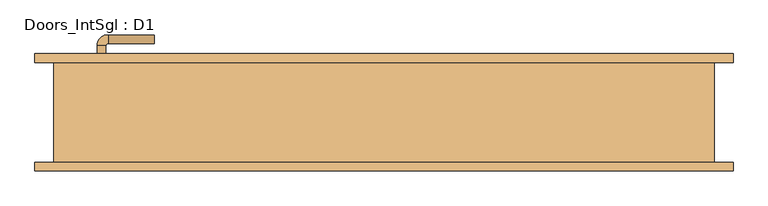
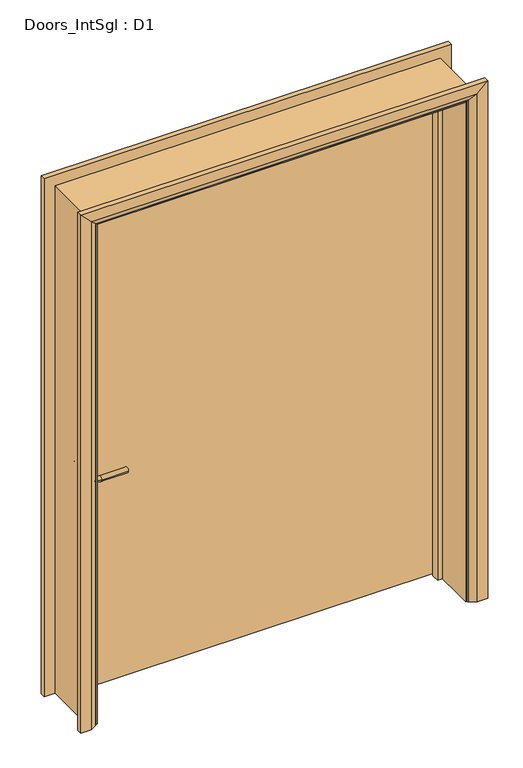
"""IFC4 building model written with IfcOpenShell, lengths in millimetres: door geometry, Doors_IntSgl : D1."""

from ifc_helpers import new_model, si_unit, point, frame, frame_2d, origin, place, context, project, spatial, polyline, circle_curve, ellipse_curve, trimmed, segment, composite_curve, outline, extrude, faceted_brep, source, transform, mapped, element, save
from ifc_brep_helpers import plane_surface, cylinder_surface, revolved_surface, advanced_brep


def doors_intsgl_d1_5c0f405e(model_context):
    return source(origin(), model_context, "Body", "SolidModel", [
        advanced_brep(
        [(-655.0, 68.3, 900.0), (-635.0, 68.3, 900.0), (-635.0, 38.3, 900.0), (-655.0, 38.3, 900.0), (-630.0, 33.3, 900.0), (-630.0, 13.3, 900.0), (-525.0, 13.3, 900.0), (-525.0, 33.3, 900.0)],
        [
            (0, 1, circle_curve(frame((-645.0, 68.3, 900.0), z_axis=(0.0, 1.0, 0.0), x_axis=(1.0, 0.0, 0.0)), 10.0)),
            (1, 0, circle_curve(frame((-645.0, 68.3, 900.0), z_axis=(0.0, 1.0, 0.0), x_axis=(1.0, 0.0, 0.0)), 10.0)),
            (1, 2),
            (2, 3, circle_curve(frame((-645.0, 38.3, 900.0), z_axis=(0.0, 1.0, 0.0), x_axis=(1.0, 0.0, 0.0)), 10.0)),
            (3, 0),
            (3, 2, circle_curve(frame((-645.0, 38.3, 900.0), z_axis=(0.0, 1.0, 0.0), x_axis=(1.0, 0.0, 0.0)), 10.0)),
            (4, 5, circle_curve(frame((-630.0, 23.3, 900.0), z_axis=(-1.0, 0.0, 0.0), x_axis=(0.0, 1.0, 0.0)), 10.0)),
            (5, 3, circle_curve(frame((-630.0, 38.3, 900.0), z_axis=(0.0, 0.0, -1.0), x_axis=(-1.0, 0.0, 0.0)), 25.0)),
            (2, 4, circle_curve(frame((-630.0, 38.3, 900.0), z_axis=(0.0, 0.0, 1.0), x_axis=(-1.0, 0.0, 0.0)), 5.0)),
            (5, 4, circle_curve(frame((-630.0, 23.3, 900.0), z_axis=(-1.0, 0.0, 0.0), x_axis=(0.0, 1.0, 0.0)), 10.0)),
            (6, 7, circle_curve(frame((-525.0, 23.3, 900.0), z_axis=(1.0, 0.0, 0.0), x_axis=(0.0, 1.0, 0.0)), 10.0)),
            (7, 6, circle_curve(frame((-525.0, 23.3, 900.0), z_axis=(1.0, 0.0, 0.0), x_axis=(0.0, 1.0, 0.0)), 10.0)),
            (4, 7),
            (6, 5),
        ],
        [
            plane_surface(frame((-645.0, 68.3, 900.0), z_axis=(0.0, 1.0, 0.0), x_axis=(0.0, 0.0, 1.0))),
            cylinder_surface(frame((-645.0, 68.3, 900.0), z_axis=(0.0, 1.0, 0.0), x_axis=(1.0, 0.0, 0.0)), 10.0),
            revolved_surface(trimmed(ellipse_curve(frame((-645.0, 38.3, 900.0), z_axis=(0.0, -1.0, 0.0), x_axis=(1.0, 0.0, 0.0)), 10.0, 10.0), [point((-655.0, 38.3, 900.0))], [point((-635.0, 38.3, 900.0))], True, "CARTESIAN"), (-630.0, 38.3, 900.0), (0.0, 0.0, -1.0)),
            revolved_surface(trimmed(ellipse_curve(frame((-645.0, 38.3, 900.0), z_axis=(0.0, -1.0, 0.0), x_axis=(1.0, 0.0, 0.0)), 10.0, 10.0), [point((-635.0, 38.3, 900.0))], [point((-655.0, 38.3, 900.0))], True, "CARTESIAN"), (-630.0, 38.3, 900.0), (0.0, 0.0, -1.0)),
            plane_surface(frame((-525.0, 23.3, 900.0), z_axis=(1.0, 0.0, 0.0), x_axis=(0.0, 0.0, 1.0))),
            cylinder_surface(frame((-630.0, 23.3, 900.0), z_axis=(-1.0, 0.0, 0.0), x_axis=(0.0, 1.0, 0.0)), 10.0),
        ],
        [
            (0, [[1, 2]]),
            (1, [[3, 4, 5, -2]]),
            (1, [[-5, 6, -3, -1]]),
            (2, [[7, 8, -4, 9]]),
            (3, [[10, -9, -6, -8]]),
            (4, [[11, 12]]),
            (5, [[13, -11, 14, -7]]),
            (5, [[-14, -12, -13, -10]]),
        ],
    ),
        extrude(outline(composite_curve([segment(trimmed(circle_curve(frame_2d((900.0, -647.5)), 30.0), [point((900.0, -677.5))], [point((900.0, -617.5))], False, "CARTESIAN"), True, "CONTINUOUS"), segment(trimmed(circle_curve(frame_2d((900.0, -647.5)), 30.0), [point((900.0, -617.5))], [point((900.0, -677.5))], False, "CARTESIAN"), True, "CONTINUOUS")], self_intersect=False)), frame((0.0, 68.3, 0.0), z_axis=(0.0, 1.0, 0.0), x_axis=(0.0, 0.0, 1.0)), (0.0, 0.0, 1.0), 8.0),
        advanced_brep(
        [(-655.0, 122.3, 900.0), (-635.0, 122.3, 900.0), (-655.0, 152.3, 900.0), (-635.0, 152.3, 900.0), (-630.0, 157.3, 900.0), (-630.0, 177.3, 900.0), (-525.0, 177.3, 900.0), (-525.0, 157.3, 900.0)],
        [
            (0, 1, circle_curve(frame((-645.0, 122.3, 900.0), z_axis=(0.0, -1.0, 0.0), x_axis=(1.0, 0.0, 0.0)), 10.0)),
            (1, 0, circle_curve(frame((-645.0, 122.3, 900.0), z_axis=(0.0, -1.0, 0.0), x_axis=(1.0, 0.0, 0.0)), 10.0)),
            (0, 2),
            (2, 3, circle_curve(frame((-645.0, 152.3, 900.0), z_axis=(0.0, -1.0, 0.0), x_axis=(1.0, 0.0, 0.0)), 10.0)),
            (3, 1),
            (3, 2, circle_curve(frame((-645.0, 152.3, 900.0), z_axis=(0.0, -1.0, 0.0), x_axis=(1.0, 0.0, 0.0)), 10.0)),
            (4, 3, circle_curve(frame((-630.0, 152.3, 900.0), z_axis=(0.0, 0.0, 1.0), x_axis=(-1.0, 0.0, 0.0)), 5.0)),
            (2, 5, circle_curve(frame((-630.0, 152.3, 900.0), z_axis=(0.0, 0.0, -1.0), x_axis=(-1.0, 0.0, 0.0)), 25.0)),
            (5, 4, circle_curve(frame((-630.0, 167.3, 900.0), z_axis=(-1.0, 0.0, 0.0), x_axis=(0.0, -1.0, 0.0)), 10.0)),
            (4, 5, circle_curve(frame((-630.0, 167.3, 900.0), z_axis=(-1.0, 0.0, 0.0), x_axis=(0.0, -1.0, 0.0)), 10.0)),
            (6, 7, circle_curve(frame((-525.0, 167.3, 900.0), z_axis=(1.0, 0.0, 0.0), x_axis=(0.0, -1.0, 0.0)), 10.0)),
            (7, 6, circle_curve(frame((-525.0, 167.3, 900.0), z_axis=(1.0, 0.0, 0.0), x_axis=(0.0, -1.0, 0.0)), 10.0)),
            (5, 6),
            (7, 4),
        ],
        [
            plane_surface(frame((-645.0, 122.3, 900.0), z_axis=(0.0, -1.0, 0.0), x_axis=(0.0, 0.0, 1.0))),
            cylinder_surface(frame((-645.0, 122.3, 900.0), z_axis=(0.0, -1.0, 0.0), x_axis=(1.0, 0.0, 0.0)), 10.0),
            revolved_surface(trimmed(ellipse_curve(frame((-645.0, 152.3, 900.0), z_axis=(0.0, -1.0, 0.0), x_axis=(1.0, 0.0, 0.0)), 10.0, 10.0), [point((-655.0, 152.3, 900.0))], [point((-635.0, 152.3, 900.0))], True, "CARTESIAN"), (-630.0, 152.3, 900.0), (0.0, 0.0, -1.0)),
            revolved_surface(trimmed(ellipse_curve(frame((-645.0, 152.3, 900.0), z_axis=(0.0, -1.0, 0.0), x_axis=(1.0, 0.0, 0.0)), 10.0, 10.0), [point((-635.0, 152.3, 900.0))], [point((-655.0, 152.3, 900.0))], True, "CARTESIAN"), (-630.0, 152.3, 900.0), (0.0, 0.0, -1.0)),
            plane_surface(frame((-525.0, 167.3, 900.0), z_axis=(1.0, 0.0, 0.0), x_axis=(0.0, 0.0, 1.0))),
            cylinder_surface(frame((-630.0, 167.3, 900.0), z_axis=(-1.0, 0.0, 0.0), x_axis=(0.0, -1.0, 0.0)), 10.0),
        ],
        [
            (0, [[1, 2]]),
            (1, [[-1, 3, 4, 5]]),
            (1, [[-2, -5, 6, -3]]),
            (2, [[7, -4, 8, 9]]),
            (3, [[-8, -6, -7, 10]]),
            (4, [[11, 12]]),
            (5, [[-9, 13, -12, 14]]),
            (5, [[-10, -14, -11, -13]]),
        ],
    ),
        extrude(outline(composite_curve([segment(trimmed(circle_curve(frame_2d((900.0, -647.5)), 30.0), [point((900.0, -677.5))], [point((900.0, -617.5))], False, "CARTESIAN"), True, "CONTINUOUS"), segment(trimmed(circle_curve(frame_2d((900.0, -647.5)), 30.0), [point((900.0, -617.5))], [point((900.0, -677.5))], False, "CARTESIAN"), True, "CONTINUOUS")], self_intersect=False)), frame((0.0, 114.3, 0.0), z_axis=(0.0, 1.0, 0.0), x_axis=(0.0, 0.0, 1.0)), (0.0, 0.0, 1.0), 8.0),
        extrude(outline(polyline([(720.0, 76.3), (-720.0, 76.3), (-720.0, 114.3), (720.0, 114.3), (720.0, 76.3)])), frame((0.0, 0.0, 8.0), z_axis=(0.0, 0.0, 1.0), x_axis=(1.0, 0.0, 0.0)), (0.0, 0.0, 1.0), 2060.0),
        advanced_brep(
        [(797.0, 134.3, 0.0), (797.0, 114.3, 0.0), (727.0, 114.3, 0.0), (731.0, 120.3, 0.0), (757.0, 134.3, 0.0), (797.0, 134.3, 2145.0), (797.0, 114.3, 2145.0), (-797.0, 114.3, 2145.0), (-797.0, 114.3, 0.0), (-727.0, 114.3, 0.0), (-727.0, 114.3, 2075.0), (727.0, 114.3, 2075.0), (731.0, 120.3, 2079.0), (757.0, 134.3, 2105.0), (-757.0, 134.3, 2105.0), (-757.0, 134.3, 0.0), (-797.0, 134.3, 0.0), (-797.0, 134.3, 2145.0), (-731.0, 120.3, 0.0), (-731.0, 120.3, 2079.0)],
        [
            (0, 1),
            (1, 2),
            (2, 3, circle_curve(frame((735.0, 113.3, 0.0), z_axis=(0.0, 0.0, -1.0), x_axis=(1.0, 0.0, 0.0)), 8.0622577)),
            (3, 4),
            (4, 0),
            (0, 5),
            (5, 6),
            (6, 1),
            (6, 7),
            (7, 8),
            (8, 9),
            (9, 10),
            (10, 11),
            (11, 2),
            (11, 12, ellipse_curve(frame((735.0, 113.3, 2083.0), z_axis=(0.7071067811865475, 0.0, -0.7071067811865475), x_axis=(-0.7071067811865474, 0.0, -0.7071067811865476)), 11.4017543, 8.0622577)),
            (12, 3),
            (12, 13),
            (13, 4),
            (13, 14),
            (14, 15),
            (15, 16),
            (16, 17),
            (17, 5),
            (7, 17),
            (16, 8),
            (15, 18),
            (18, 9, circle_curve(frame((-735.0, 113.3, 0.0), z_axis=(0.0, 0.0, -1.0), x_axis=(-1.0, 0.0, 0.0)), 8.0622577)),
            (19, 10, ellipse_curve(frame((-735.0, 113.3, 2083.0), z_axis=(-0.7071067811865475, 0.0, -0.7071067811865475), x_axis=(-0.7071067811865474, 0.0, 0.7071067811865476)), 11.4017543, 8.0622577)),
            (18, 19),
            (14, 19),
            (19, 12),
        ],
        [
            plane_surface(frame((727.0, 114.3, 0.0), z_axis=(0.0, 0.0, -1.0), x_axis=(0.0, -1.0, 0.0))),
            plane_surface(frame((797.0, 134.3, 0.0), z_axis=(1.0, 0.0, 0.0), x_axis=(0.0, 0.0, 1.0))),
            plane_surface(frame((797.0, 114.3, 0.0), z_axis=(0.0, -1.0, 0.0), x_axis=(0.0, 0.0, 1.0))),
            cylinder_surface(frame((735.0, 113.3, 0.0), z_axis=(0.0, 0.0, -1.0), x_axis=(1.0, 0.0, 0.0)), 8.0622577),
            plane_surface(frame((731.0, 120.3, 0.0), z_axis=(-0.4740998230350126, 0.880471099922178, 0.0), x_axis=(0.0, 0.0, 1.0))),
            plane_surface(frame((757.0, 134.3, 0.0), z_axis=(0.0, 1.0, 0.0), x_axis=(0.0, 0.0, 1.0))),
            plane_surface(frame((-797.0, 134.3, 2145.0), z_axis=(-1.0, 0.0, 0.0), x_axis=(0.0, 0.0, -1.0))),
            plane_surface(frame((-727.0, 114.3, 0.0), z_axis=(0.0, 0.0, -1.0), x_axis=(0.0, -1.0, 0.0))),
            cylinder_surface(frame((-735.0, 113.3, 2075.0), z_axis=(0.0, 0.0, 1.0), x_axis=(-1.0, 0.0, 0.0)), 8.0622577),
            plane_surface(frame((-731.0, 120.3, 2079.0), z_axis=(0.47409982303501824, 0.8804710999221749, 0.0), x_axis=(0.0, 0.0, -1.0))),
            plane_surface(frame((797.0, 134.3, 2145.0), z_axis=(0.0, 0.0, 1.0), x_axis=(-1.0, 0.0, 0.0))),
            cylinder_surface(frame((727.0, 113.3, 2083.0), z_axis=(1.0, 0.0, 0.0), x_axis=(0.0, 0.0, 1.0)), 8.0622577),
            plane_surface(frame((731.0, 120.3, 2079.0), z_axis=(0.0, 0.8804710999221764, -0.4740998230350154), x_axis=(-1.0, 0.0, 0.0))),
        ],
        [
            (0, [[1, 2, 3, 4, 5]]),
            (1, [[-1, 6, 7, 8]]),
            (2, [[-2, -8, 9, 10, 11, 12, 13, 14]]),
            (3, [[-3, -14, 15, 16]]),
            (4, [[-4, -16, 17, 18]]),
            (5, [[-5, -18, 19, 20, 21, 22, 23, -6]]),
            (6, [[24, -22, 25, -10]]),
            (7, [[-21, 26, 27, -11, -25]]),
            (8, [[28, -12, -27, 29]]),
            (9, [[30, -29, -26, -20]]),
            (10, [[-7, -23, -24, -9]]),
            (11, [[-15, -13, -28, 31]]),
            (12, [[-17, -31, -30, -19]]),
        ],
    ),
        extrude(outline(polyline([(0.0, -722.0), (0.0, -703.0), (2051.0, -703.0), (2051.0, 703.0), (0.0, 703.0), (0.0, 722.0), (2070.0, 722.0), (2070.0, -722.0), (0.0, -722.0)])), frame((0.0, 42.3, 0.0), z_axis=(0.0, 1.0, 0.0), x_axis=(0.0, 0.0, 1.0)), (0.0, 0.0, 1.0), 32.0),
        advanced_brep(
        [(-797.0, -134.3, 0.0), (-797.0, -114.3, 0.0), (-727.0, -114.3, 0.0), (-731.0, -120.3, 0.0), (-757.0, -134.3, 0.0), (-797.0, -134.3, 2145.0), (-797.0, -114.3, 2145.0), (-727.0, -114.3, 2075.0), (-731.0, -120.3, 2079.0), (-757.0, -134.3, 2105.0), (797.0, -134.3, 0.0), (757.0, -134.3, 0.0), (731.0, -120.3, 0.0), (727.0, -114.3, 0.0), (797.0, -114.3, 0.0), (797.0, -134.3, 2145.0), (757.0, -134.3, 2105.0), (731.0, -120.3, 2079.0), (727.0, -114.3, 2075.0), (797.0, -114.3, 2145.0)],
        [
            (0, 1),
            (1, 2),
            (2, 3, circle_curve(frame((-735.0, -113.3, 0.0), z_axis=(0.0, 0.0, -1.0), x_axis=(-1.0, 0.0, 0.0)), 8.0622577)),
            (3, 4),
            (4, 0),
            (0, 5),
            (5, 6),
            (6, 1),
            (6, 7),
            (7, 2),
            (7, 8, ellipse_curve(frame((-735.0, -113.3, 2083.0), z_axis=(-0.7071067811865475, 0.0, -0.7071067811865475), x_axis=(0.7071067811865474, 0.0, -0.7071067811865476)), 11.4017543, 8.0622577)),
            (8, 3),
            (8, 9),
            (9, 4),
            (9, 5),
            (10, 11),
            (11, 12),
            (12, 13, circle_curve(frame((735.0, -113.3, 0.0), z_axis=(0.0, 0.0, -1.0), x_axis=(1.0, 0.0, 0.0)), 8.0622577)),
            (13, 14),
            (14, 10),
            (15, 16),
            (16, 11),
            (10, 15),
            (16, 17),
            (17, 12),
            (17, 18, ellipse_curve(frame((735.0, -113.3, 2083.0), z_axis=(0.7071067811865475, 0.0, -0.7071067811865475), x_axis=(0.7071067811865474, 0.0, 0.7071067811865476)), 11.4017543, 8.0622577)),
            (18, 13),
            (18, 19),
            (19, 14),
            (19, 15),
            (5, 15),
            (19, 6),
            (18, 7),
            (17, 8),
            (16, 9),
        ],
        [
            plane_surface(frame((-727.0, -187.1010989, 0.0), z_axis=(0.0, 0.0, -1.0), x_axis=(1.0, 0.0, 0.0))),
            plane_surface(frame((-797.0, -134.3, 0.0), z_axis=(-1.0, 0.0, 0.0), x_axis=(0.0, 0.0, 1.0))),
            plane_surface(frame((-797.0, -114.3, 0.0), z_axis=(0.0, 1.0, 0.0), x_axis=(0.0, 0.0, 1.0))),
            cylinder_surface(frame((-735.0, -113.3, 0.0), z_axis=(0.0, 0.0, -1.0), x_axis=(-1.0, 0.0, 0.0)), 8.0622577),
            plane_surface(frame((-731.0, -120.3, 0.0), z_axis=(0.4740998230350183, -0.8804710999221749, 0.0), x_axis=(0.0, 0.0, 1.0))),
            plane_surface(frame((-757.0, -134.3, 0.0), z_axis=(0.0, -1.0, 0.0), x_axis=(0.0, 0.0, 1.0))),
            plane_surface(frame((727.0, -187.1010989, 0.0), z_axis=(0.0, 0.0, -1.0), x_axis=(-1.0, 0.0, 0.0))),
            plane_surface(frame((757.0, -134.3, 2105.0), z_axis=(0.0, -1.0, 0.0), x_axis=(0.0, 0.0, -1.0))),
            plane_surface(frame((731.0, -120.3, 2079.0), z_axis=(-0.4740998230350183, -0.8804710999221749, 0.0), x_axis=(0.0, 0.0, -1.0))),
            cylinder_surface(frame((735.0, -113.3, 2075.0), z_axis=(0.0, 0.0, 1.0), x_axis=(1.0, 0.0, 0.0)), 8.0622577),
            plane_surface(frame((797.0, -114.3, 2145.0), z_axis=(0.0, 1.0, 0.0), x_axis=(0.0, 0.0, -1.0))),
            plane_surface(frame((797.0, -134.3, 2145.0), z_axis=(1.0, 0.0, 0.0), x_axis=(0.0, 0.0, -1.0))),
            plane_surface(frame((-797.0, -134.3, 2145.0), z_axis=(0.0, 0.0, 1.0), x_axis=(1.0, 0.0, 0.0))),
            plane_surface(frame((-797.0, -114.3, 2145.0), z_axis=(0.0, 1.0, 0.0), x_axis=(1.0, 0.0, 0.0))),
            cylinder_surface(frame((-727.0, -113.3, 2083.0), z_axis=(-1.0, 0.0, 0.0), x_axis=(0.0, 0.0, 1.0)), 8.0622577),
            plane_surface(frame((-731.0, -120.3, 2079.0), z_axis=(0.0, -0.8804710999221749, -0.4740998230350183), x_axis=(1.0, 0.0, 0.0))),
            plane_surface(frame((-757.0, -134.3, 2105.0), z_axis=(0.0, -1.0, 0.0), x_axis=(1.0, 0.0, 0.0))),
        ],
        [
            (0, [[1, 2, 3, 4, 5]]),
            (1, [[-1, 6, 7, 8]]),
            (2, [[-2, -8, 9, 10]]),
            (3, [[-3, -10, 11, 12]]),
            (4, [[-4, -12, 13, 14]]),
            (5, [[-5, -14, 15, -6]]),
            (6, [[16, 17, 18, 19, 20]]),
            (7, [[21, 22, -16, 23]]),
            (8, [[24, 25, -17, -22]]),
            (9, [[26, 27, -18, -25]]),
            (10, [[28, 29, -19, -27]]),
            (11, [[30, -23, -20, -29]]),
            (12, [[-7, 31, -30, 32]]),
            (13, [[-9, -32, -28, 33]]),
            (14, [[-11, -33, -26, 34]]),
            (15, [[-13, -34, -24, 35]]),
            (16, [[-15, -35, -21, -31]]),
        ],
    ),
        faceted_brep([(-722.0, 114.3, 0.0), (-722.0, -114.3, 0.0), (-754.0, -114.3, 0.0), (-754.0, 114.3, 0.0), (-722.0, 114.3, 2070.0), (-722.0, -114.3, 2070.0), (-754.0, -114.3, 2102.0), (-754.0, 114.3, 2102.0), (722.0, 114.3, 0.0), (754.0, 114.3, 0.0), (754.0, -114.3, 0.0), (722.0, -114.3, 0.0), (722.0, 114.3, 2070.0), (754.0, 114.3, 2102.0), (754.0, -114.3, 2102.0), (722.0, -114.3, 2070.0)], [[[0, 1, 2, 3]], [[1, 0, 4, 5]], [[2, 1, 5, 6]], [[3, 2, 6, 7]], [[0, 3, 7, 4]], [[8, 9, 10, 11]], [[12, 13, 9, 8]], [[13, 14, 10, 9]], [[14, 15, 11, 10]], [[15, 12, 8, 11]], [[5, 4, 12, 15]], [[6, 5, 15, 14]], [[7, 6, 14, 13]], [[4, 7, 13, 12]]]),
    ])


if __name__ == "__main__":
    model = new_model("IFC4")
    model_context = context("Model", 3, world=origin())
    ifc_project = project(units=[si_unit("LENGTHUNIT", "METRE", prefix="MILLI")], contexts=[model_context])
    site = spatial("IfcSite", under=ifc_project)
    building = spatial("IfcBuilding", under=site)
    placement = place(None, origin())
    doors_intsgl_d1_shape = doors_intsgl_d1_5c0f405e(model_context)
    element("IfcDoor", 1, ObjectType="Doors_IntSgl : D1", at=placement, inside=building, context=model_context, shape_type="MappedRepresentation", body=[
        mapped(doors_intsgl_d1_shape, transform((0.0, 0.0, 0.0), x_axis=(1.0, 0.0, 0.0), y_axis=(0.0, 1.0, 0.0), z_axis=(0.0, 0.0, 1.0))),
    ])
    save(model, "model.ifc")

# Revit data of these elements
# Type "Doors_IntSgl : D1"
#   Type Mark = "46"
#   Type Comments = "Internal Single"
#   Operation = "SingleSwingRight"
#   Manufacturer = "Revit"
#   Keynote = "L20"
#   Description = "Internal Single Door"
#   Analytic Construction = "Metal"
#   UnderCut = 8 mm
#   Tolerance = 2 mm
#   Thickness = 38 mm
#   Thermal Resistance (R) = 0.270117 (m²·K)/W
#   Structural Tolerance = 8 mm
#   StopDepth = 32 mm
#   Stop Thickness = 19 mm
#   Rough Width = 1524 mm
#   Rough Height = 2110 mm
#   Height to Top Lock Rail = 1000 mm
#   Heat Transfer Coefficient (U) = 3.7021 W/(m²·K)
#   Handle Z Distance = 900 mm
#   Handle X Distance = 75 mm
#   Frame Thickness = 32 mm
#   Door Panel Width = 1440 mm
#   Door Panel Thickness = 38 mm
#   Door Panel Offset = 0 mm
#   Height = 2110 mm
#   Width = 1524 mm
#   Door Panel Height = 2060 mm
#   Architrave Setback = 5 mm
#   Vis - Ironmongery = yes
#   Material Ironmongery = Door - Handle
#   Material Frame = Door - Frame/Mullion (1)
#   Material Door = Door - Panel
#   Material Architrave = Door - Architrave
#   Visual Light Transmittance = 0
#   Solar Heat Gain Coefficient = 0
#   Function = (empty or 0)
#   Wall Closure = (empty or 0)
# Element 1 (IfcDoor, "Doors_IntSgl : D1")
#   Materials on its faces: "Door - Architrave", "Door - Handle", "Door - Frame/Mullion (1)", "Door - Panel"
# Materials
#   "Door - Handle": colour RGB 0 0 0, transparency 0, Keynote = "P21", Cost = 0
#   "Door - Frame/Mullion (1)": class "Wood", colour RGB 212 179 113, transparency 0, Keynote = "L20", Cost = 0
#   "Door - Panel": class "Wood", colour RGB 210 159 95, transparency 0, Keynote = "L20", Cost = 0
#   "Door - Architrave": class "Wood", colour RGB 154 90 5, transparency 0, Keynote = "P20", Cost = 0
